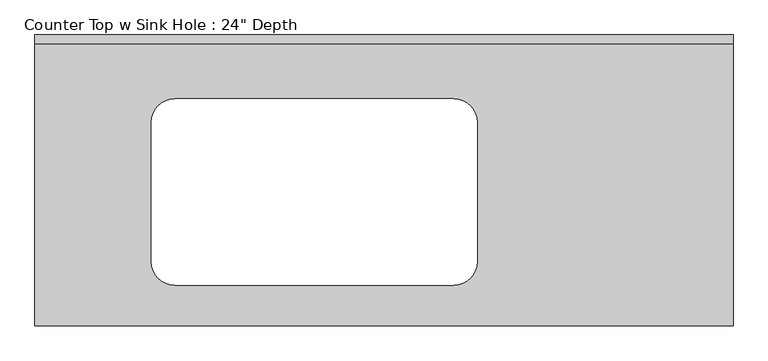
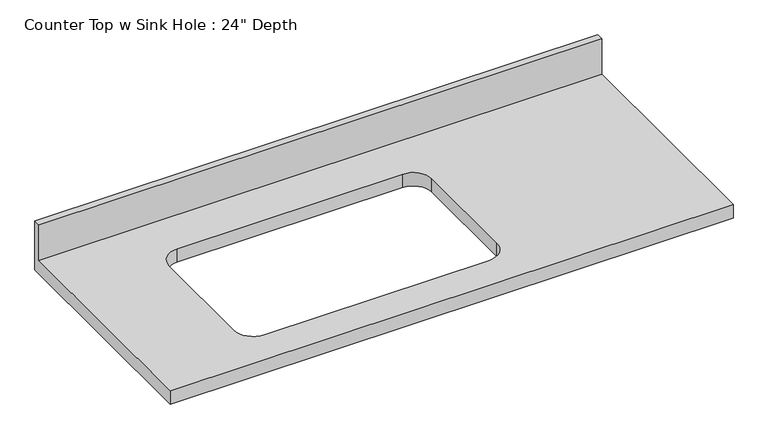
"""IFC4 building model written with IfcOpenShell, lengths in millimetres: furniture geometry."""

from ifc_helpers import new_model, si_unit, frame, origin, place, context, project, spatial, polyline, circle_curve, source, transform, mapped, element, save
from ifc_brep_helpers import plane_surface, revolved_surface, advanced_brep


def furniture_6430aa70(model_context):
    return source(origin(), model_context, "Body", "AdvancedBrep", [
        advanced_brep(
        [(-1200.4622951, -635.0, 914.4), (323.5377049, -635.0, 914.4), (323.5377049, -19.05, 914.4), (-1200.4622951, -19.05, 914.4), (-895.6622951, -139.7, 914.4), (-286.0622951, -139.7, 914.4), (-235.2622951, -190.5, 914.4), (-235.2622951, -495.3, 914.4), (-286.0622951, -546.1, 914.4), (-895.6622951, -546.1, 914.4), (-946.4622951, -495.3, 914.4), (-946.4622951, -190.5, 914.4), (323.5377049, 0.0, 876.3), (323.5377049, -635.0, 876.3), (-1200.4622951, -635.0, 876.3), (-1200.4622951, 0.0, 876.3), (-286.0622951, -139.7, 876.3), (-895.6622951, -139.7, 876.3), (-946.4622951, -190.5, 876.3), (-946.4622951, -495.3, 876.3), (-895.6622951, -546.1, 876.3), (-286.0622951, -546.1, 876.3), (-235.2622951, -495.3, 876.3), (-235.2622951, -190.5, 876.3), (-1200.4622951, 0.0, 1016.0), (323.5377049, 0.0, 1016.0), (-1200.4622951, -19.05, 1016.0), (323.5377049, -19.05, 1016.0)],
        [
            (0, 1),
            (1, 2),
            (2, 3),
            (3, 0),
            (4, 5),
            (5, 6, circle_curve(frame((-286.0622951, -190.5, 914.4), z_axis=(0.0, 0.0, -1.0), x_axis=(1.0, 0.0, 0.0)), 50.8)),
            (6, 7),
            (7, 8, circle_curve(frame((-286.0622951, -495.3, 914.4), z_axis=(0.0, 0.0, -1.0), x_axis=(1.0, 0.0, 0.0)), 50.8)),
            (8, 9),
            (9, 10, circle_curve(frame((-895.6622951, -495.3, 914.4), z_axis=(0.0, 0.0, -1.0), x_axis=(1.0, 0.0, 0.0)), 50.8)),
            (10, 11),
            (11, 4, circle_curve(frame((-895.6622951, -190.5, 914.4), z_axis=(0.0, 0.0, -1.0), x_axis=(1.0, 0.0, 0.0)), 50.8)),
            (12, 13),
            (13, 14),
            (14, 15),
            (15, 12),
            (16, 17),
            (17, 18, circle_curve(frame((-895.6622951, -190.5, 876.3), z_axis=(0.0, 0.0, 1.0), x_axis=(1.0, 0.0, 0.0)), 50.8)),
            (18, 19),
            (19, 20, circle_curve(frame((-895.6622951, -495.3, 876.3), z_axis=(0.0, 0.0, 1.0), x_axis=(1.0, 0.0, 0.0)), 50.8)),
            (20, 21),
            (21, 22, circle_curve(frame((-286.0622951, -495.3, 876.3), z_axis=(0.0, 0.0, 1.0), x_axis=(1.0, 0.0, 0.0)), 50.8)),
            (22, 23),
            (23, 16, circle_curve(frame((-286.0622951, -190.5, 876.3), z_axis=(0.0, 0.0, 1.0), x_axis=(1.0, 0.0, 0.0)), 50.8)),
            (15, 24),
            (24, 25),
            (25, 12),
            (14, 0),
            (3, 26),
            (26, 24),
            (13, 1),
            (25, 27),
            (27, 2),
            (4, 17),
            (16, 5),
            (11, 18),
            (10, 19),
            (9, 20),
            (8, 21),
            (7, 22),
            (6, 23),
            (26, 27),
        ],
        [
            plane_surface(frame((-1200.4622951, 0.0, 914.4), z_axis=(0.0, 0.0, 1.0), x_axis=(-1.0, 0.0, 0.0))),
            plane_surface(frame((-1200.4622951, 0.0, 876.3), z_axis=(0.0, 0.0, -1.0), x_axis=(1.0, 0.0, 0.0))),
            plane_surface(frame((323.5377049, 0.0, 914.4), z_axis=(0.0, 1.0, 0.0), x_axis=(0.0, 0.0, -1.0))),
            plane_surface(frame((-1200.4622951, 0.0, 914.4), z_axis=(-1.0, 0.0, 0.0), x_axis=(0.0, 0.0, -1.0))),
            plane_surface(frame((-1200.4622951, -635.0, 914.4), z_axis=(0.0, -1.0, 0.0), x_axis=(0.0, 0.0, -1.0))),
            plane_surface(frame((323.5377049, -635.0, 914.4), z_axis=(1.0, 0.0, 0.0), x_axis=(0.0, 0.0, -1.0))),
            plane_surface(frame((-286.0622951, -139.7, 914.4), z_axis=(0.0, -1.0, 0.0), x_axis=(0.0, 0.0, -1.0))),
            revolved_surface(polyline([(-844.8622951000001, -190.5, 914.4), (-844.8622951000001, -190.5, 876.3)]), (-895.6622951, -190.5, 876.3), (0.0, 0.0, 1.0)),
            plane_surface(frame((-946.4622951, -190.5, 914.4), z_axis=(1.0, 0.0, 0.0), x_axis=(0.0, 0.0, -1.0))),
            revolved_surface(polyline([(-844.8622951000001, -495.3, 914.4), (-844.8622951000001, -495.3, 876.3)]), (-895.6622951, -495.3, 876.3), (0.0, 0.0, 1.0)),
            plane_surface(frame((-895.6622951, -546.1, 914.4), z_axis=(0.0, 1.0, 0.0), x_axis=(0.0, 0.0, -1.0))),
            revolved_surface(polyline([(-235.26229509999996, -495.3, 914.4), (-235.26229509999996, -495.3, 876.3)]), (-286.0622951, -495.3, 876.3), (0.0, 0.0, 1.0)),
            plane_surface(frame((-235.2622951, -495.3, 914.4), z_axis=(-1.0, 0.0, 0.0), x_axis=(0.0, 0.0, -1.0))),
            revolved_surface(polyline([(-235.26229509999996, -190.5, 914.4), (-235.26229509999996, -190.5, 876.3)]), (-286.0622951, -190.5, 876.3), (0.0, 0.0, 1.0)),
            plane_surface(frame((-1200.4622951, 0.0, 1016.0), z_axis=(0.0, 0.0, 1.0), x_axis=(0.0, -1.0, 0.0))),
            plane_surface(frame((-1200.4622951, -19.05, 1016.0), z_axis=(0.0, -1.0, 0.0), x_axis=(0.0, 0.0, -1.0))),
        ],
        [
            (0, [[1, 2, 3, 4], [5, 6, 7, 8, 9, 10, 11, 12]]),
            (1, [[13, 14, 15, 16], [17, 18, 19, 20, 21, 22, 23, 24]]),
            (2, [[-16, 25, 26, 27]]),
            (3, [[-15, 28, -4, 29, 30, -25]]),
            (4, [[-1, -28, -14, 31]]),
            (5, [[-13, -27, 32, 33, -2, -31]]),
            (6, [[34, -17, 35, -5]]),
            (7, [[-34, -12, 36, -18]]),
            (8, [[-36, -11, 37, -19]]),
            (9, [[-37, -10, 38, -20]]),
            (10, [[-38, -9, 39, -21]]),
            (11, [[-39, -8, 40, -22]]),
            (12, [[-40, -7, 41, -23]]),
            (13, [[-35, -24, -41, -6]]),
            (14, [[-30, 42, -32, -26]]),
            (15, [[-42, -29, -3, -33]]),
        ],
    ),
    ])


if __name__ == "__main__":
    model = new_model("IFC4")
    model_context = context("Model", 3, world=origin())
    ifc_project = project(units=[si_unit("LENGTHUNIT", "METRE", prefix="MILLI")], contexts=[model_context])
    site = spatial("IfcSite", under=ifc_project)
    building = spatial("IfcBuilding", under=site)
    placement = place(None, origin())
    furniture_shape = furniture_6430aa70(model_context)
    element("IfcFurniture", 1, ObjectType="Counter Top w Sink Hole : 24\" Depth", at=placement, inside=building, context=model_context, shape_type="MappedRepresentation", body=[
        mapped(furniture_shape, transform((0.0, 0.0, 0.0), x_axis=(1.0, 0.0, 0.0), y_axis=(0.0, 1.0, 0.0), z_axis=(0.0, 0.0, 1.0))),
    ])
    save(model, "model.ifc")

# Revit data of these elements
# Type "Counter Top w Sink Hole : 24\" Depth"
#   Assembly Code = "C1030400"
#   Counter Thickness = 0' - 1 1/2"
#   Depth = 2' - 1"
#   Height = 3' - 0"
#   Length [instance default] = 8' - 0"
#   Sink Location [instance default] = 2' - 0"
#   Sink Location To Wall [instance default] = 0' - 6"
#   Sink Opening Depth [instance default] = 1' - 3"
#   Sink Opening Width [instance default] = 2' - 3"
#   Counter Top Material = none
#   Default Elevation = 0
# Element 1 (IfcFurniture, "Counter Top w Sink Hole : 24\" Depth")
#   Length = 5' - 0"
#   Materials on its faces: "Counter Top"
# Materials
#   "Counter Top": class "Wood", colour RGB 226 177 128, transparency 0
